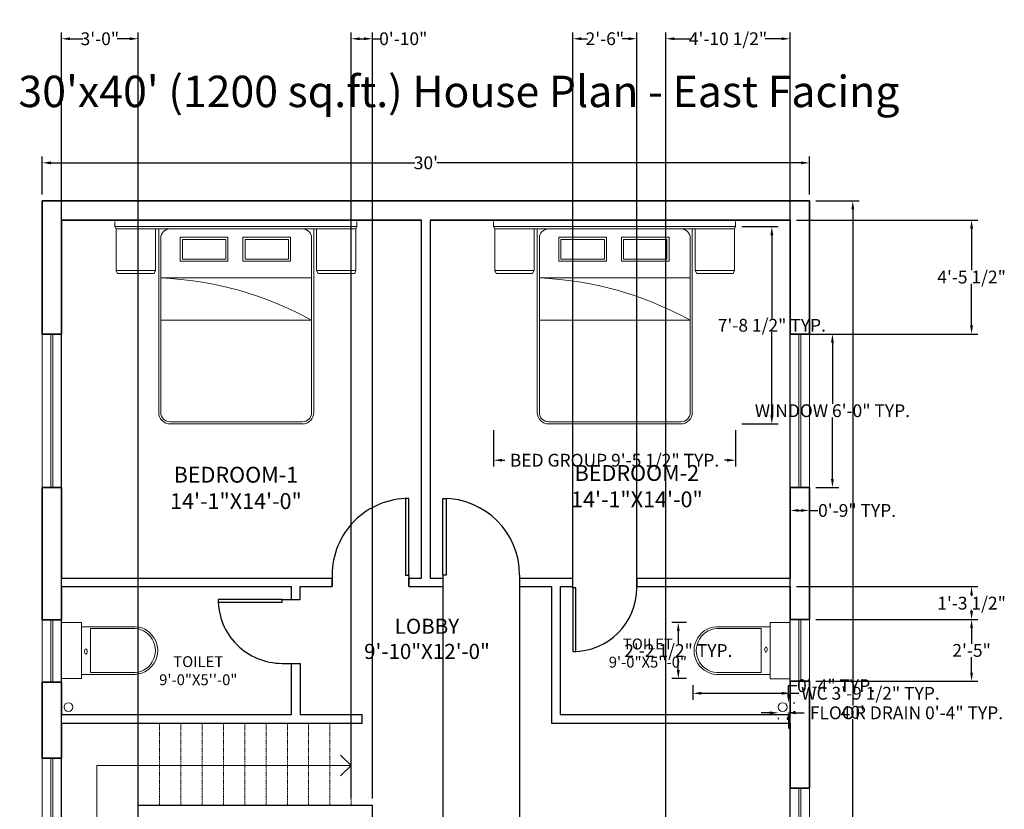
# Model space of a CAD drawing. Units: inches. Extents: x 328 to 872, y 288 to 933.
# Tile 2 of 2: x 410 to 872, y 562 to 933. Entities that reach past the tile are written whole.
import ezdxf

# ---------------------------------------------------------------- set-up
doc = ezdxf.new("R2010")
doc.units = ezdxf.units.IN
doc.header["$MEASUREMENT"] = 0
doc.linetypes.add('DASHED', pattern=[0.75, 0.5, -0.25])
for name, color, linetype, lineweight in [('A-ANNO-DIMS', 2, 'Continuous', 18), ('A-ANNO-SYMB', 7, 'Continuous', 18), ('A-ANNO-TEXT', 7, 'Continuous', 18), ('A-AREA-IDEN', 7, 'Continuous', 18), ('A-FLOR-FIXT', 11, 'Continuous', 18), ('A-FLOR-STRS-OVHD', 30, 'DASHED', 18), ('Commode', 203, 'Continuous', 18), ('Doors', 28, 'Continuous', 25), ('Furniture', 90, 'Continuous', 18), ('Inner Wall', 14, 'Continuous', 30), ('Outer Wall', 10, 'Continuous', 35), ('Stairs', 30, 'Continuous', 25), ('Ventilators', 140, 'Continuous', 18), ('Windows', 160, 'Continuous', 18)]:
    doc.layers.add(name, color=color, linetype=linetype, lineweight=lineweight)
doc.styles.get("Standard").update_dxf_attribs({"font": 'arial.ttf'})
doc.dimstyles.get("Standard").update_dxf_attribs({"dimtxt": 6, "dimasz": 4, "dimexe": 3, "dimexo": 3, "dimgap": 0.09, "dimtad": 0, "dimtih": 1, "dimtoh": 1, "dimdec": 1, "dimzin": 0, "dimdsep": 46, "dimlunit": 3, "dimtxsty": 'Standard', "dimcen": 0.09, "dimadec": 0, "dimazin": 0, "dimtfac": 1, "dimtdec": 1, "dimtofl": 0, "dimtmove": 0, "dimatfit": 3, "dimfxl": 1, "dimtolj": 1, "dimtzin": 0, "dimarcsym": 0})

# ---------------------------------------------------------------- blocks, each defined once
blk = doc.blocks.new('A$C6F7C6EE8')
for p, q in [((0.0287, 2.7315), (1.888, 2.7315)), ((0.0401, 2.7112), (0.0287, 2.7315)), ((2.2616, 2.7315), (1.888, 2.7315)), ((2.2513, 2.7125), (2.2616, 2.7315)), ((0.0401, 2.7112), (0.0401, 2.3265)), ((2.2513, 2.7112), (0.0401, 2.7112)), ((0.4034, 2.3265), (0.4034, 2.7112)), ((0.4322, 2.7112), (0.4322, 1.0165)), ((1.8625, 1.0165), (1.8625, 2.7112)), ((1.8893, 2.3265), (1.888, 2.7112)), ((2.2513, 2.7125), (2.2526, 2.3277)), ((0.4515, 2.6253), (0.4515, 1.0165)), ((1.8433, 1.0165), (1.8433, 2.6253)), ((0.0401, 2.3265), (0.4034, 2.3265)), ((0.0401, 2.3265), (0.0522, 2.2985)), ((0.0522, 2.2985), (0.3897, 2.2985)), ((0.4034, 2.3265), (0.3897, 2.2985)), ((2.2526, 2.3277), (1.8893, 2.3265)), ((1.8893, 2.3265), (1.9031, 2.2985)), ((2.2405, 2.2997), (1.9031, 2.2985)), ((2.2526, 2.3277), (2.2405, 2.2997)), ((0.4515, 2.2578), (1.8433, 2.2578)), ((0.4515, 1.8676), (1.8433, 1.8676)), ((0.5374, 0.9306), (1.7574, 0.9306)), ((0.5374, 0.9114), (1.7574, 0.9114))]:
    blk.add_line(p, q)
for points in [[(1.0712, 2.6336), (1.0712, 2.4115), (0.6311, 2.4115), (0.6311, 2.6336)], [(1.0512, 2.6136), (1.0512, 2.4315), (0.6511, 2.4315), (0.6511, 2.6136)], [(1.649, 2.6336), (1.649, 2.4115), (1.209, 2.4115), (1.209, 2.6336)], [(1.629, 2.6136), (1.629, 2.4315), (1.229, 2.4315), (1.229, 2.6136)]]:
    blk.add_lwpolyline(points, close=True)
for centre, radius, start, end in [((0.5374, 2.6253), 0.0859, 90, 180), ((1.7574, 2.6253), 0.0859, 0, 90), ((0.3261, -0.8662), 3.1266, 60.97174, 87.70269), ((0.5374, 1.0165), 0.1052, 180, 270), ((0.5374, 1.0165), 0.0859, 180, 270), ((1.7574, 1.0165), 0.1052, 270, 0), ((1.7574, 1.0165), 0.0859, 270, 0)]:
    blk.add_arc(centre, radius, start, end)
blk = doc.blocks.new('commod')
for p, q in [((990.3, 724), (1372.7, 724)), ((990.3, 724), (990.3, 587.3)), ((1372.7, 724), (1372.7, 587.3)), ((1372.7, 587.3), (990.3, 587.3)), ((1019.3, 587.3), (1019.3, 544.7)), ((1019.3, 544.7), (1019.3, 244.7)), ((1343.7, 587.3), (1343.7, 544.7)), ((1343.7, 544.7), (1343.7, 244.7)), ((1331.7, 527.3), (1031.3, 527.3)), ((1031.3, 527.3), (1031.3, 244.7)), ((1331.7, 527.3), (1331.7, 244.7))]:
    blk.add_line(p, q)
for centre, radius, start, end in [((1181.5, 232.6), 162.7, 175.73096, 4.26904), ((1181.5, 235.7), 150.5, 176.54415, 3.45585)]:
    blk.add_arc(centre, radius, start, end)
blk.add_ellipse((1174.8, 559), major_axis=(-16.8, 0), ratio=0.543379)
blk = doc.blocks.new('*U8')
for p, q in [((0, 0), (0, 6)), ((40, 0), (40, 6))]:
    blk.add_line(p, q)
blk.add_lwpolyline([(0, 0), (0, -40), (1.75, -40), (1.75, 0)], close=True)
blk.add_arc((0, 0), 40, 270, 0)
blk = doc.blocks.new('*U10')
for p, q in [((0, 0), (0, -6)), ((40, 0), (40, -6))]:
    blk.add_line(p, q)
blk.add_lwpolyline([(0, 0), (0, 40), (1.75, 40), (1.75, 0)], close=True)
blk.add_arc((0, 0), 40, 0, 90)
blk = doc.blocks.new('*U9')
for p, q in [((0, 0), (0, 6)), ((40, 0), (40, 6))]:
    blk.add_line(p, q)
blk.add_lwpolyline([(0, 0), (0, -40), (1.75, -40), (1.75, 0)], close=True)
blk.add_arc((0, 0), 40, 270, 0)
blk = doc.blocks.new('*D11')
at = {"layer": 'A-ANNO-DIMS', "color": 0, "lineweight": -2, "transparency": 16777216}
for p, q in [((420.12, 850.8), (420.12, 868.67)), ((424.12, 865.67), (594.94, 865.67)), ((776.12, 865.67), (605.3, 865.67)), ((780.12, 850.8), (780.12, 868.67))]:
    blk.add_line(p, q, dxfattribs=at)
at = {"layer": 'A-ANNO-DIMS', "color": 0, "transparency": 16777216}
for points in [[(424.12, 866.34), (424.12, 865), (420.12, 865.67)], [(776.12, 866.34), (776.12, 865), (780.12, 865.67)]]:
    blk.add_solid(points, dxfattribs=at)
at = {"layer": 'Defpoints', "color": 0, "transparency": 16777216}
for p in [(780.12, 865.67), (420.12, 847.8), (780.12, 847.8)]:
    blk.add_point(p, dxfattribs=at)
at = {"layer": 'A-ANNO-DIMS', "color": 0, "transparency": 16777216, "insert": (600.12, 865.67), "char_height": 6, "attachment_point": 5}
blk.add_mtext("\\A1;30'", dxfattribs=at)
blk = doc.blocks.new('*D12')
at = {"layer": 'A-ANNO-DIMS', "color": 0, "lineweight": -2, "transparency": 16777216}
for p, q in [((783.12, 847.8), (803.48, 847.8)), ((800.48, 843.8), (800.48, 610.95)), ((800.48, 371.8), (800.48, 604.65)), ((783.12, 367.8), (803.48, 367.8))]:
    blk.add_line(p, q, dxfattribs=at)
at = {"layer": 'A-ANNO-DIMS', "color": 0, "transparency": 16777216}
for points in [[(799.82, 843.8), (801.15, 843.8), (800.48, 847.8)], [(799.82, 371.8), (801.15, 371.8), (800.48, 367.8)]]:
    blk.add_solid(points, dxfattribs=at)
at = {"layer": 'Defpoints', "color": 0, "transparency": 16777216}
for p in [(780.12, 847.8), (780.12, 367.8), (800.48, 367.8)]:
    blk.add_point(p, dxfattribs=at)
at = {"layer": 'A-ANNO-DIMS', "color": 0, "transparency": 16777216, "insert": (800.48, 607.8), "char_height": 6, "attachment_point": 5}
blk.add_mtext("\\A1;40'", dxfattribs=at)
blk = doc.blocks.new('WIN-48IN')
for p, q in [((4, 0), (4, 48)), ((5, 48), (5, 0))]:
    blk.add_line(p, q)
blk.add_lwpolyline([(9, 0), (0, 0), (0, 48), (9, 48)], close=True)
blk = doc.blocks.new('WIN-72IN')
for p, q in [((4, 72), (4, 0)), ((5, 72), (5, 0))]:
    blk.add_line(p, q)
blk.add_lwpolyline([(9, 72), (9, 0), (0, 0), (0, 72)], close=True)
blk = doc.blocks.new('FLOOR-DRAIN')
blk.add_circle((2.07, 2.07), 2.07)
blk = doc.blocks.new('*D19')
at = {"layer": 'A-ANNO-DIMS', "color": 0, "lineweight": -2, "transparency": 16777216}
for p, q in [((783.12, 785.35), (793.92, 785.35)), ((790.92, 781.35), (790.92, 752.55)), ((790.92, 717.35), (790.92, 746.16)), ((783.12, 713.35), (793.92, 713.35))]:
    blk.add_line(p, q, dxfattribs=at)
at = {"layer": 'A-ANNO-DIMS', "color": 0, "transparency": 16777216}
for points in [[(790.26, 781.35), (791.59, 781.35), (790.92, 785.35)], [(790.26, 717.35), (791.59, 717.35), (790.92, 713.35)]]:
    blk.add_solid(points, dxfattribs=at)
at = {"layer": 'Defpoints', "color": 0, "transparency": 16777216}
for p in [(780.12, 785.35), (790.92, 785.35), (780.12, 713.35)]:
    blk.add_point(p, dxfattribs=at)
at = {"layer": 'A-ANNO-DIMS', "color": 0, "transparency": 16777216, "insert": (790.92, 749.35), "char_height": 6, "attachment_point": 5}
blk.add_mtext('\\A1;WINDOW 6\'-0" TYP.', dxfattribs=at)
blk = doc.blocks.new('*D20')
at = {"layer": 'A-ANNO-DIMS', "color": 0, "lineweight": -2, "transparency": 16777216}
for p, q in [((771.12, 710.35), (771.12, 699.55)), ((780.12, 710.35), (780.12, 699.55)), ((775.12, 702.55), (776.12, 702.55)), ((780.12, 702.55), (784.12, 702.55))]:
    blk.add_line(p, q, dxfattribs=at)
at = {"layer": 'A-ANNO-DIMS', "color": 0, "transparency": 16777216}
for points in [[(775.12, 703.22), (775.12, 701.89), (771.12, 702.55)], [(776.12, 703.22), (776.12, 701.89), (780.12, 702.55)]]:
    blk.add_solid(points, dxfattribs=at)
at = {"layer": 'Defpoints', "color": 0, "transparency": 16777216}
for p in [(771.12, 713.35), (780.12, 713.35), (780.12, 702.55)]:
    blk.add_point(p, dxfattribs=at)
at = {"layer": 'A-ANNO-DIMS', "color": 0, "transparency": 16777216, "insert": (802.5, 702.55), "char_height": 6, "attachment_point": 5}
blk.add_mtext('\\A1;0\'-9" TYP.', dxfattribs=at)
blk = doc.blocks.new('*D21')
at = {"layer": 'A-ANNO-DIMS', "color": 0, "lineweight": -2, "transparency": 16777216}
for p, q in [((631.88, 740.16), (631.88, 723.12)), ((745.46, 740.16), (745.46, 723.12)), ((635.88, 726.12), (637.12, 726.12)), ((741.46, 726.12), (740.22, 726.12))]:
    blk.add_line(p, q, dxfattribs=at)
at = {"layer": 'A-ANNO-DIMS', "color": 0, "transparency": 16777216}
for points in [[(635.88, 726.79), (635.88, 725.45), (631.88, 726.12)], [(741.46, 726.79), (741.46, 725.45), (745.46, 726.12)]]:
    blk.add_solid(points, dxfattribs=at)
at = {"layer": 'Defpoints', "color": 0, "transparency": 16777216}
for p in [(631.88, 743.16), (745.46, 743.16), (745.46, 726.12)]:
    blk.add_point(p, dxfattribs=at)
at = {"layer": 'A-ANNO-DIMS', "color": 0, "transparency": 16777216, "insert": (688.67, 726.12), "char_height": 6, "attachment_point": 5}
blk.add_mtext('\\A1;BED GROUP 9\'-5 1/2" TYP.', dxfattribs=at)
blk = doc.blocks.new('*D22')
at = {"layer": 'A-ANNO-DIMS', "color": 0, "lineweight": -2, "transparency": 16777216}
for p, q in [((748.46, 835.73), (765.49, 835.73)), ((762.49, 831.73), (762.49, 792.64)), ((762.49, 747.16), (762.49, 786.25)), ((748.46, 743.16), (765.49, 743.16))]:
    blk.add_line(p, q, dxfattribs=at)
at = {"layer": 'A-ANNO-DIMS', "color": 0, "transparency": 16777216}
for points in [[(761.82, 831.73), (763.16, 831.73), (762.49, 835.73)], [(761.82, 747.16), (763.16, 747.16), (762.49, 743.16)]]:
    blk.add_solid(points, dxfattribs=at)
at = {"layer": 'Defpoints', "color": 0, "transparency": 16777216}
for p in [(745.46, 835.73), (762.49, 835.73), (745.46, 743.16)]:
    blk.add_point(p, dxfattribs=at)
at = {"layer": 'A-ANNO-DIMS', "color": 0, "transparency": 16777216, "insert": (762.49, 789.45), "char_height": 6, "attachment_point": 5}
blk.add_mtext('\\A1;7\'-8 1/2" TYP.', dxfattribs=at)
blk = doc.blocks.new('*D23')
at = {"layer": 'A-ANNO-DIMS', "color": 0, "lineweight": -2, "transparency": 16777216}
for p, q in [((725.44, 620.61), (725.44, 613.75)), ((771.12, 620.61), (771.12, 613.75)), ((729.44, 616.75), (767.12, 616.75)), ((771.12, 616.75), (775.12, 616.75))]:
    blk.add_line(p, q, dxfattribs=at)
at = {"layer": 'A-ANNO-DIMS', "color": 0, "transparency": 16777216}
for points in [[(729.44, 617.42), (729.44, 616.09), (725.44, 616.75)], [(767.12, 617.42), (767.12, 616.09), (771.12, 616.75)]]:
    blk.add_solid(points, dxfattribs=at)
at = {"layer": 'Defpoints', "color": 0, "transparency": 16777216}
for p in [(725.44, 623.61), (771.12, 623.61), (771.12, 616.75)]:
    blk.add_point(p, dxfattribs=at)
at = {"layer": 'A-ANNO-DIMS', "color": 0, "transparency": 16777216, "insert": (808.76, 616.75), "char_height": 6, "attachment_point": 5}
blk.add_mtext('\\A1;WC 3\'-9 1/2" TYP.', dxfattribs=at)
blk = doc.blocks.new('*D24')
at = {"layer": 'A-ANNO-DIMS', "color": 0, "lineweight": -2, "transparency": 16777216}
for p, q in [((722.44, 650), (715.59, 650)), ((718.59, 646), (718.59, 639.99)), ((718.59, 627.61), (718.59, 633.61)), ((722.44, 623.61), (715.59, 623.61))]:
    blk.add_line(p, q, dxfattribs=at)
at = {"layer": 'A-ANNO-DIMS', "color": 0, "transparency": 16777216}
for points in [[(717.92, 646), (719.25, 646), (718.59, 650)], [(717.92, 627.61), (719.25, 627.61), (718.59, 623.61)]]:
    blk.add_solid(points, dxfattribs=at)
at = {"layer": 'Defpoints', "color": 0, "transparency": 16777216}
for p in [(725.44, 650), (718.59, 623.61), (725.44, 623.61)]:
    blk.add_point(p, dxfattribs=at)
at = {"layer": 'A-ANNO-DIMS', "color": 0, "transparency": 16777216, "insert": (718.59, 636.8), "char_height": 6, "attachment_point": 5}
blk.add_mtext('\\A1;2\'-2 1/2" TYP.', dxfattribs=at)
blk = doc.blocks.new('*D25')
at = {"layer": 'A-ANNO-DIMS', "color": 0, "lineweight": -2, "transparency": 16777216}
for p, q in [((761.52, 607.58), (757.52, 607.58)), ((773.66, 607.58), (777.66, 607.58)), ((765.52, 605.2), (765.52, 604.58)), ((769.66, 605.2), (769.66, 604.58))]:
    blk.add_line(p, q, dxfattribs=at)
at = {"layer": 'A-ANNO-DIMS', "color": 0, "transparency": 16777216}
for points in [[(761.52, 608.24), (761.52, 606.91), (765.52, 607.58)], [(773.66, 608.24), (773.66, 606.91), (769.66, 607.58)]]:
    blk.add_solid(points, dxfattribs=at)
at = {"layer": 'Defpoints', "color": 0, "transparency": 16777216}
for p in [(765.52, 608.2), (769.66, 608.2), (769.66, 607.58)]:
    blk.add_point(p, dxfattribs=at)
at = {"layer": 'A-ANNO-DIMS', "color": 0, "transparency": 16777216, "insert": (825.67, 607.58), "char_height": 6, "attachment_point": 5}
blk.add_mtext('\\A1;FLOOR DRAIN 0\'-4" TYP.', dxfattribs=at)
blk = doc.blocks.new('*D26')
at = {"layer": 'A-ANNO-DIMS', "color": 0, "lineweight": -2, "transparency": 16777216}
for p, q in [((770.28, 616.33), (770.28, 620.33)), ((770.28, 620.33), (774.28, 620.33)), ((772.66, 612.33), (773.28, 612.33)), ((772.66, 608.2), (773.28, 608.2)), ((770.28, 604.2), (770.28, 600.2))]:
    blk.add_line(p, q, dxfattribs=at)
at = {"layer": 'A-ANNO-DIMS', "color": 0, "transparency": 16777216}
for points in [[(769.61, 616.33), (770.94, 616.33), (770.28, 612.33)], [(769.61, 604.2), (770.94, 604.2), (770.28, 608.2)]]:
    blk.add_solid(points, dxfattribs=at)
at = {"layer": 'Defpoints', "color": 0, "transparency": 16777216}
for p in [(769.66, 612.33), (770.28, 612.33), (769.66, 608.2)]:
    blk.add_point(p, dxfattribs=at)
at = {"layer": 'A-ANNO-DIMS', "color": 0, "transparency": 16777216, "insert": (792.65, 620.33), "char_height": 6, "attachment_point": 5}
blk.add_mtext('\\A1;0\'-4" TYP.', dxfattribs=at)
blk = doc.blocks.new('*D35')
at = {"layer": 'A-ANNO-DIMS', "color": 0, "lineweight": -2, "transparency": 16777216}
for p, q in [((712.72, 423.18), (712.72, 926.91)), ((771.12, 423.18), (771.12, 926.91)), ((716.72, 923.91), (724.42, 923.91)), ((767.12, 923.91), (759.43, 923.91))]:
    blk.add_line(p, q, dxfattribs=at)
at = {"layer": 'A-ANNO-DIMS', "color": 0, "transparency": 16777216}
for points in [[(716.72, 924.57), (716.72, 923.24), (712.72, 923.91)], [(767.12, 924.57), (767.12, 923.24), (771.12, 923.91)]]:
    blk.add_solid(points, dxfattribs=at)
at = {"layer": 'Defpoints', "color": 0, "transparency": 16777216}
for p in [(771.12, 923.91), (712.72, 420.18), (771.12, 420.18)]:
    blk.add_point(p, dxfattribs=at)
at = {"layer": 'A-ANNO-DIMS', "color": 0, "transparency": 16777216, "insert": (741.92, 923.91), "char_height": 6, "attachment_point": 5}
blk.add_mtext('\\A1;4\'-10 1/2"', dxfattribs=at)
blk = doc.blocks.new('*D37')
at = {"layer": 'A-ANNO-DIMS', "color": 0, "lineweight": -2, "transparency": 16777216}
for p, q in [((608.12, 667.8), (608.12, 288.7)), ((644.12, 667.8), (644.12, 288.7)), ((612.12, 291.7), (618.06, 291.7)), ((640.12, 291.7), (634.19, 291.7))]:
    blk.add_line(p, q, dxfattribs=at)
at = {"layer": 'A-ANNO-DIMS', "color": 0, "transparency": 16777216}
for points in [[(612.12, 292.36), (612.12, 291.03), (608.12, 291.7)], [(640.12, 292.36), (640.12, 291.03), (644.12, 291.7)]]:
    blk.add_solid(points, dxfattribs=at)
at = {"layer": 'Defpoints', "color": 0, "transparency": 16777216}
for p in [(608.12, 670.8), (644.12, 670.8), (644.12, 291.7)]:
    blk.add_point(p, dxfattribs=at)
at = {"layer": 'A-ANNO-DIMS', "color": 0, "transparency": 16777216, "insert": (626.12, 291.7), "char_height": 6, "attachment_point": 5}
blk.add_mtext('\\A1;3\'-0"', dxfattribs=at)
blk = doc.blocks.new('*D38')
at = {"layer": 'A-ANNO-DIMS', "color": 0, "lineweight": -2, "transparency": 16777216}
for p, q in [((669.12, 669.8), (669.12, 926.91)), ((699.12, 669.8), (699.12, 926.91)), ((673.12, 923.91), (676.01, 923.91)), ((695.12, 923.91), (692.24, 923.91))]:
    blk.add_line(p, q, dxfattribs=at)
at = {"layer": 'A-ANNO-DIMS', "color": 0, "transparency": 16777216}
for points in [[(673.12, 924.57), (673.12, 923.24), (669.12, 923.91)], [(695.12, 924.57), (695.12, 923.24), (699.12, 923.91)]]:
    blk.add_solid(points, dxfattribs=at)
at = {"layer": 'Defpoints', "color": 0, "transparency": 16777216}
for p in [(699.12, 923.91), (669.12, 666.8), (699.12, 666.8)]:
    blk.add_point(p, dxfattribs=at)
at = {"layer": 'A-ANNO-DIMS', "color": 0, "transparency": 16777216, "insert": (684.12, 923.91), "char_height": 6, "attachment_point": 5}
blk.add_mtext('\\A1;2\'-6"', dxfattribs=at)
blk = doc.blocks.new('*D39')
at = {"layer": 'A-ANNO-DIMS', "color": 0, "lineweight": -2, "transparency": 16777216}
for p, q in [((774.12, 838.8), (859.23, 838.8)), ((856.23, 834.8), (856.23, 815.27)), ((856.23, 789.35), (856.23, 808.88)), ((774.12, 785.35), (859.23, 785.35))]:
    blk.add_line(p, q, dxfattribs=at)
at = {"layer": 'A-ANNO-DIMS', "color": 0, "transparency": 16777216}
for points in [[(855.56, 834.8), (856.89, 834.8), (856.23, 838.8)], [(855.56, 789.35), (856.89, 789.35), (856.23, 785.35)]]:
    blk.add_solid(points, dxfattribs=at)
at = {"layer": 'Defpoints', "color": 0, "transparency": 16777216}
for p in [(771.12, 838.8), (856.23, 838.8), (771.12, 785.35)]:
    blk.add_point(p, dxfattribs=at)
at = {"layer": 'A-ANNO-DIMS', "color": 0, "transparency": 16777216, "insert": (856.23, 812.08), "char_height": 6, "attachment_point": 5}
blk.add_mtext('\\A1;4\'-5 1/2"', dxfattribs=at)
blk = doc.blocks.new('*D43')
at = {"layer": 'A-ANNO-DIMS', "color": 0, "lineweight": -2, "transparency": 16777216}
for p, q in [((429.12, 524.8), (429.12, 926.91)), ((465.12, 524.8), (465.12, 926.91)), ((433.12, 923.91), (439.06, 923.91)), ((461.12, 923.91), (455.19, 923.91))]:
    blk.add_line(p, q, dxfattribs=at)
at = {"layer": 'A-ANNO-DIMS', "color": 0, "transparency": 16777216}
for points in [[(433.12, 924.57), (433.12, 923.24), (429.12, 923.91)], [(461.12, 924.57), (461.12, 923.24), (465.12, 923.91)]]:
    blk.add_solid(points, dxfattribs=at)
at = {"layer": 'Defpoints', "color": 0, "transparency": 16777216}
for p in [(465.12, 923.91), (429.12, 521.8), (465.12, 521.8)]:
    blk.add_point(p, dxfattribs=at)
at = {"layer": 'A-ANNO-DIMS', "color": 0, "transparency": 16777216, "insert": (447.12, 923.91), "char_height": 6, "attachment_point": 5}
blk.add_mtext('\\A1;3\'-0"', dxfattribs=at)
blk = doc.blocks.new('*D46')
at = {"layer": 'A-ANNO-DIMS', "color": 0, "lineweight": -2, "transparency": 16777216}
for p, q in [((565.12, 567.3), (565.12, 926.91)), ((575.12, 567.3), (575.12, 926.91)), ((569.12, 923.91), (571.12, 923.91)), ((575.12, 923.91), (579.12, 923.91))]:
    blk.add_line(p, q, dxfattribs=at)
at = {"layer": 'A-ANNO-DIMS', "color": 0, "transparency": 16777216}
for points in [[(569.12, 924.57), (569.12, 923.24), (565.12, 923.91)], [(571.12, 924.57), (571.12, 923.24), (575.12, 923.91)]]:
    blk.add_solid(points, dxfattribs=at)
at = {"layer": 'Defpoints', "color": 0, "transparency": 16777216}
for p in [(575.12, 923.91), (565.12, 564.3), (575.12, 564.3)]:
    blk.add_point(p, dxfattribs=at)
at = {"layer": 'A-ANNO-DIMS', "color": 0, "transparency": 16777216, "insert": (589.52, 923.91), "char_height": 6, "attachment_point": 5}
blk.add_mtext('\\A1;0\'-10"', dxfattribs=at)
blk = doc.blocks.new('*D47')
at = {"layer": 'A-ANNO-DIMS', "color": 0, "lineweight": -2, "transparency": 16777216}
for p, q in [((783.12, 651.31), (859.23, 651.31)), ((856.23, 647.31), (856.23, 640.03)), ((856.23, 626.44), (856.23, 633.72)), ((783.12, 622.44), (859.23, 622.44))]:
    blk.add_line(p, q, dxfattribs=at)
at = {"layer": 'A-ANNO-DIMS', "color": 0, "transparency": 16777216}
for points in [[(855.56, 647.31), (856.89, 647.31), (856.23, 651.31)], [(855.56, 626.44), (856.89, 626.44), (856.23, 622.44)]]:
    blk.add_solid(points, dxfattribs=at)
at = {"layer": 'Defpoints', "color": 0, "transparency": 16777216}
for p in [(780.12, 651.31), (856.23, 651.31), (780.12, 622.44)]:
    blk.add_point(p, dxfattribs=at)
at = {"layer": 'A-ANNO-DIMS', "color": 0, "transparency": 16777216, "insert": (856.23, 636.87), "char_height": 6, "attachment_point": 5}
blk.add_mtext('\\A1;2\'-5"', dxfattribs=at)
blk = doc.blocks.new('*D48')
at = {"layer": 'A-ANNO-DIMS', "color": 0, "lineweight": -2, "transparency": 16777216}
for p, q in [((774.12, 666.8), (859.23, 666.8)), ((856.23, 662.8), (856.23, 662.25)), ((856.23, 655.31), (856.23, 655.86)), ((783.12, 651.31), (859.23, 651.31))]:
    blk.add_line(p, q, dxfattribs=at)
at = {"layer": 'A-ANNO-DIMS', "color": 0, "transparency": 16777216}
for points in [[(855.56, 662.8), (856.89, 662.8), (856.23, 666.8)], [(855.56, 655.31), (856.89, 655.31), (856.23, 651.31)]]:
    blk.add_solid(points, dxfattribs=at)
at = {"layer": 'Defpoints', "color": 0, "transparency": 16777216}
for p in [(771.12, 666.8), (856.23, 666.8), (780.12, 651.31)]:
    blk.add_point(p, dxfattribs=at)
at = {"layer": 'A-ANNO-DIMS', "color": 0, "transparency": 16777216, "insert": (856.23, 659.05), "char_height": 6, "attachment_point": 5}
blk.add_mtext('\\A1;1\'-3 1/2"', dxfattribs=at)

msp = doc.modelspace()

# ---------------------------------------------------------------- linework, layer by layer
at = {"layer": 'A-ANNO-SYMB'}
for p, q in [((565.12, 582.8), (560, 587.66)), ((445.67, 540.02), (445.67, 582.8)), ((445.67, 582.8), (565.12, 582.8)), ((565.12, 582.8), (560, 577.94))]:
    msp.add_line(p, q, dxfattribs=at)
at = {"layer": 'A-FLOR-STRS-OVHD'}
for p, q in [((465.12, 521.8), (465.12, 602.8)), ((475.12, 564.3), (475.12, 602.8)), ((485.12, 564.3), (485.12, 602.8)), ((495.12, 564.3), (495.12, 602.8)), ((505.12, 564.3), (505.12, 602.8)), ((515.12, 564.3), (515.12, 602.8)), ((525.12, 564.3), (525.12, 602.8)), ((535.12, 564.3), (535.12, 602.8)), ((545.12, 564.3), (545.12, 602.8)), ((555.12, 564.3), (555.12, 602.8)), ((565.12, 564.3), (565.12, 602.8))]:
    msp.add_line(p, q, dxfattribs=at)
at = {"layer": 'Commode'}
msp.add_line((429.12, 623.61), (429.12, 650), dxfattribs=at)
at = {"layer": 'Furniture'}
for p, q in [((454.21, 835.73), (454.21, 838.13)), ((567.78, 835.73), (567.78, 838.13)), ((631.88, 835.73), (631.88, 838.13)), ((745.46, 835.73), (745.46, 838.13))]:
    msp.add_line(p, q, dxfattribs=at)
at = {"layer": 'Inner Wall'}
for p, q in [((598.12, 670.8), (598.12, 838.8)), ((602.12, 838.8), (602.12, 670.8)), ((429.12, 670.8), (556.12, 670.8)), ((429.12, 670.8), (556.12, 670.8)), ((556.12, 666.8), (556.12, 670.8)), ((592.12, 666.8), (592.12, 670.8)), ((592.12, 670.8), (598.12, 670.8)), ((592.12, 670.8), (598.12, 670.8)), ((602.12, 670.8), (608.12, 670.8)), ((608.12, 670.8), (608.12, 666.8)), ((644.12, 670.8), (644.12, 666.8)), ((644.12, 670.8), (669.12, 670.8)), ((699.12, 670.8), (699.12, 666.8)), ((699.12, 670.8), (771.12, 670.8)), ((699.12, 670.8), (771.12, 670.8)), ((429.12, 666.8), (537.12, 666.8)), ((537.12, 660.8), (537.12, 666.8)), ((541.12, 666.8), (556.12, 666.8)), ((541.12, 660.8), (541.12, 666.8)), ((592.12, 666.8), (608.12, 666.8)), ((644.12, 666.8), (659.12, 666.8)), ((659.12, 666.8), (659.12, 602.8)), ((663.12, 666.8), (663.12, 606.8)), ((663.12, 666.8), (669.12, 666.8)), ((699.12, 666.8), (771.12, 666.8)), ((537.12, 660.8), (541.12, 660.8)), ((537.12, 606.8), (537.12, 630.8)), ((537.12, 630.8), (541.12, 630.8)), ((541.12, 630.8), (541.12, 606.8)), ((429.12, 606.8), (537.12, 606.8)), ((541.12, 606.8), (570.26, 606.8)), ((570.26, 602.8), (570.26, 606.8)), ((663.12, 606.8), (771.12, 606.8)), ((429.12, 602.8), (570.26, 602.8)), ((659.12, 602.8), (771.12, 602.8))]:
    msp.add_line(p, q, dxfattribs=at)
at = {"layer": 'Outer Wall'}
for p, q in [((429.12, 838.8), (598.12, 838.8)), ((429.12, 785.35), (429.12, 838.8)), ((602.12, 838.8), (771.12, 838.8)), ((771.12, 838.8), (771.12, 785.35)), ((429.12, 785.35), (420.12, 785.35)), ((771.12, 785.35), (780.12, 785.35)), ((429.12, 713.35), (420.12, 713.35)), ((429.12, 670.8), (429.12, 713.35)), ((771.12, 713.35), (780.12, 713.35)), ((771.12, 713.35), (771.12, 670.8)), ((429.12, 651.22), (429.12, 666.8)), ((771.12, 666.8), (771.12, 651.31)), ((429.12, 651.22), (420.12, 651.22)), ((771.12, 651.31), (780.12, 651.31)), ((429.12, 622), (420.12, 622)), ((429.12, 606.8), (429.12, 622)), ((771.12, 622.44), (780.12, 622.44)), ((771.12, 622.44), (771.12, 606.8)), ((429.12, 586.36), (429.12, 602.8)), ((771.12, 602.8), (771.12, 572.17)), ((429.12, 586.36), (420.12, 586.36)), ((771.12, 572.17), (780.12, 572.17))]:
    msp.add_line(p, q, dxfattribs=at)
for points in [[(420.12, 785.35), (420.12, 847.8), (780.12, 847.8), (780.12, 785.35)], [(420.12, 651.22), (420.12, 713.35)], [(780.12, 713.35), (780.12, 651.31)], [(420.12, 586.36), (420.12, 622)], [(420.12, 586.36), (420.12, 622)], [(780.12, 622.44), (780.12, 572.17)]]:
    msp.add_lwpolyline(points, dxfattribs=at)
at = {"layer": 'Stairs'}
for p in [(465.12, 564.3), (575.12, 521.8)]:
    msp.add_line(p, (575.12, 564.3), dxfattribs=at)
at = {"layer": 'Ventilators'}
for p, q in [((424.12, 622), (424.12, 651.22)), ((425.12, 651.22), (425.12, 622)), ((775.12, 622.41), (775.12, 651.31)), ((776.12, 651.31), (776.12, 622.41))]:
    msp.add_line(p, q, dxfattribs=at)
for points in [[(429.12, 651.22), (429.12, 622), (420.12, 622), (420.12, 651.22)], [(780.12, 622.41), (771.12, 622.41), (771.12, 651.31), (780.12, 651.31)]]:
    msp.add_lwpolyline(points, close=True, dxfattribs=at)

# ---------------------------------------------------------------- block references
at = {"layer": 'A-FLOR-FIXT'}
for p in [(430.3, 608.2), (765.52, 608.2)]:
    msp.add_blockref('FLOOR-DRAIN', p, dxfattribs=at)
at = {"layer": 'Commode', "xscale": 0.0690085382552883, "yscale": 0.0690085382552883, "zscale": 0.0690085382552883}
for p, rotation in [((479.09, 555.27), 89.99999999997551), ((721.16, 718.33), 269.9999999999755)]:
    msp.add_blockref('commod', p, dxfattribs=dict(at, rotation=rotation))
at = {"layer": 'Doors'}
for p, xscale, yscale, zscale, rotation in [((592.12, 672.2), 0.9, 0.9, 0.9, 180), ((532.62, 660.8), 0.75, 0.75, 0.75, 270.0000000000002)]:
    msp.add_blockref('*U9', p, dxfattribs=dict(at, xscale=xscale, yscale=yscale, zscale=zscale, rotation=rotation))
for name, p, xscale, yscale, zscale in [('*U10', (608.12, 672.2), 0.9, 0.9, 0.9), ('*U8', (669.12, 666.3), 0.749999999999994, 0.749999999999994, 0.749999999999994)]:
    msp.add_blockref(name, p, dxfattribs=dict(at, xscale=xscale, yscale=yscale, zscale=zscale))
at = {"layer": 'Furniture', "xscale": 50.86410320426389, "yscale": 50.86410320426389, "zscale": 50.86410320426389}
for p in [(452.75, 696.8), (630.42, 696.8)]:
    msp.add_blockref('A$C6F7C6EE8', p, dxfattribs=at)
at = {"layer": 'Windows'}
for name, p in [('WIN-72IN', (420.12, 713.35)), ('WIN-72IN', (771.12, 713.35)), ('WIN-48IN', (420.12, 538.36)), ('WIN-48IN', (771.12, 524.17))]:
    msp.add_blockref(name, p, dxfattribs=at)

# ---------------------------------------------------------------- texts
at = {"layer": 'A-ANNO-TEXT', "insert": (-877.72, 906.56), "char_height": 14.7445, "attachment_point": 1}
msp.add_mtext_dynamic_manual_height_columns("\\pxqc;{\\fArial|b1|i0|c0|p34;30'x40' (1200 sq.ft.) House Plan - East Facing}", width=2986.7435, gutter_width=73.72, heights=[0], dxfattribs=at)
at = {"layer": 'A-AREA-IDEN', "attachment_point": 1}
for s, width, gutter_width, insert, char_height in [('\\pxqc;BEDROOM-1\\P14\'-1"X14\'-0"', 1504.1481, 37.13, (-241.09, 723.03), 7.4254), ('\\pxqc;BEDROOM-2\\P14\'-1"X14\'-0"', 1504.1481, 37.13, (-52.92, 723.84), 7.4254), ('\\pxqc;LOBBY\\P9\'-10"X12\'-0"', 1434.9763, 35.42, (-116.85, 651.75), 7.084), ('\\pxqc;TOILET\\P9\'-0"X5\'\'-0"', 1034.2942, 25.53, (187.17, 642.43), 5.1059), ('\\pxqc;TOILET\\P9\'-0"X5\'\'-0"', 1034.2942, 25.53, (-23.83, 634.16), 5.1059)]:
    msp.add_mtext_dynamic_manual_height_columns(s, width=width, gutter_width=gutter_width, heights=[0], dxfattribs=dict(at, insert=insert, char_height=char_height))

# ---------------------------------------------------------------- dimensions: what is measured, and where the dimension line sits
at = {"layer": 'A-ANNO-DIMS'}
for base, p1, p2, override, picture, middle in [((771.12, 923.91), (712.72, 420.18), (771.12, 420.18), {"dimdec": 1, "dimlfac": 1, "dimrnd": 0, "dimzin": 1, "dimdsep": 46, "dimlunit": 4, "dimfrac": 2}, '*D35', (741.92, 923.91)), ((465.12, 923.91), (429.12, 521.8), (465.12, 521.8), {"dimdec": 1, "dimlfac": 1, "dimrnd": 0, "dimzin": 1, "dimdsep": 46, "dimlunit": 4, "dimfrac": 2}, '*D43', (447.12, 923.91)), ((575.12, 923.91), (565.12, 564.3), (575.12, 564.3), {"dimdec": 1, "dimlfac": 1, "dimrnd": 0, "dimzin": 1, "dimdsep": 46, "dimlunit": 4, "dimfrac": 2}, '*D46', (589.52, 923.91)), ((699.12, 923.91), (669.12, 666.8), (699.12, 666.8), {"dimdec": 1, "dimlfac": 1, "dimrnd": 0, "dimzin": 1, "dimdsep": 46, "dimlunit": 4, "dimfrac": 2}, '*D38', (684.12, 923.91)), ((780.12, 865.67), (420.12, 847.8), (780.12, 847.8), {"dimclrd": 0, "dimclre": 0, "dimclrt": 0}, '*D11', (600.12, 865.67)), ((644.12, 291.7), (608.12, 670.8), (644.12, 670.8), {"dimdec": 1, "dimlfac": 1, "dimrnd": 0, "dimzin": 1, "dimdsep": 46, "dimlunit": 4, "dimfrac": 2}, '*D37', (626.12, 291.7))]:
    dim = msp.add_linear_dim(base=base, p1=p1, p2=p2, dimstyle='Standard', override=override, dxfattribs=at)
    dim.commit()
    dim.dimension.update_dxf_attribs({"geometry": picture, "text_midpoint": middle})
for base, p1, p2, override, picture, middle in [((800.48, 367.8), (780.12, 847.8), (780.12, 367.8), {"dimclrd": 0, "dimclre": 0, "dimclrt": 0}, '*D12', (800.48, 607.8)), ((856.2278, 838.8007), (771.1228, 785.3522), (771.1228, 838.8007), {"dimdec": 1, "dimlfac": 1, "dimrnd": 0, "dimzin": 1, "dimdsep": 46, "dimlunit": 4, "dimfrac": 2}, '*D39', (856.2278, 812.0765)), ((856.23, 666.8), (780.12, 651.31), (771.12, 666.8), {"dimdec": 1, "dimlfac": 1, "dimrnd": 0, "dimzin": 1, "dimdsep": 46, "dimlunit": 4, "dimfrac": 2}, '*D48', (856.23, 659.05)), ((856.23, 651.31), (780.12, 622.44), (780.12, 651.31), {"dimdec": 1, "dimlfac": 1, "dimrnd": 0, "dimzin": 1, "dimdsep": 46, "dimlunit": 4, "dimfrac": 2}, '*D47', (856.23, 636.87))]:
    dim = msp.add_linear_dim(base=base, p1=p1, p2=p2, angle=90, dimstyle='Standard', override=override, dxfattribs=at)
    dim.commit()
    dim.dimension.update_dxf_attribs({"geometry": picture, "text_midpoint": middle})
for base, p1, p2, angle, text, picture, middle in [((762.49, 835.73), (745.46, 743.16), (745.46, 835.73), 90, '<> TYP.', '*D22', (762.49, 789.45)), ((790.92, 785.35), (780.12, 713.35), (780.12, 785.35), 90, 'WINDOW <> TYP.', '*D19', (790.92, 749.35)), ((718.59, 623.61), (725.44, 650), (725.44, 623.61), 270, '<> TYP.', '*D24', (718.59, 636.8)), ((770.28, 612.33), (769.66, 608.2), (769.66, 612.33), 90, '<> TYP.', '*D26', (792.65, 620.33))]:
    dim = msp.add_linear_dim(base=base, p1=p1, p2=p2, angle=angle, text=text, dimstyle='Standard', override={"dimdec": 1, "dimlfac": 1, "dimrnd": 0, "dimzin": 1, "dimdsep": 46, "dimlunit": 4, "dimfrac": 2}, dxfattribs=at)
    dim.commit()
    dim.dimension.update_dxf_attribs({"geometry": picture, "text_midpoint": middle})
for base, p1, p2, text, picture, middle in [((745.46, 726.12), (631.88, 743.16), (745.46, 743.16), 'BED GROUP <> TYP.', '*D21', (688.67, 726.12)), ((780.12, 702.55), (771.12, 713.35), (780.12, 713.35), '<> TYP.', '*D20', (802.5, 702.55)), ((771.12, 616.75), (725.44, 623.61), (771.12, 623.61), 'WC <> TYP.', '*D23', (808.76, 616.75)), ((769.66, 607.58), (765.52, 608.2), (769.66, 608.2), 'FLOOR DRAIN <> TYP.', '*D25', (825.67, 607.58))]:
    dim = msp.add_linear_dim(base=base, p1=p1, p2=p2, text=text, dimstyle='Standard', override={"dimdec": 1, "dimlfac": 1, "dimrnd": 0, "dimzin": 1, "dimdsep": 46, "dimlunit": 4, "dimfrac": 2}, dxfattribs=at)
    dim.commit()
    dim.dimension.update_dxf_attribs({"geometry": picture, "text_midpoint": middle})

doc.saveas('drawing.dxf')
